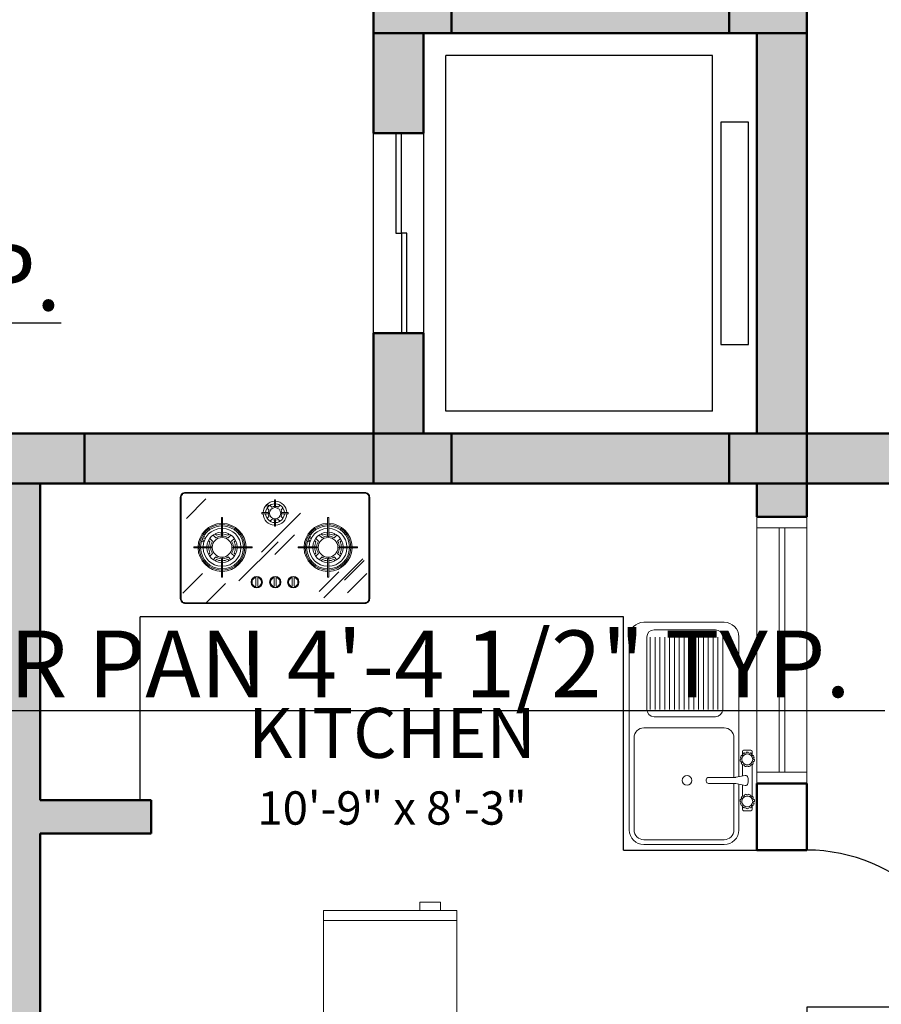
# Model space of a CAD drawing. Units: inches. Extents: x 375 to 1122, y 27 to 1069.
# Tile 79 of 155: x 790 to 945, y 400 to 577. Entities that reach past the tile are written whole.
import ezdxf

# ---------------------------------------------------------------- set-up
doc = ezdxf.new("R2010")
doc.units = ezdxf.units.IN
for name, color, linetype, lineweight in [('A-ANNO-DIMS', 2, 'Continuous', 18), ('A-AREA-IDEN', 7, 'Continuous', 18), ('A-COLS-PATT', 10, 'Continuous', 13), ('A-EQPM', 55, 'Continuous', 18), ('A-FLOR-EVTR', 40, 'Continuous', 25), ('A-FLOR-FIXT', 55, 'Continuous', 18), ('A-FLOR-MILL', 55, 'Continuous', 25), ('A-WALL-PATT', 252, 'Continuous', 13), ('Columns', 10, 'Continuous', 50), ('Doors', 150, 'Continuous', 25), ('Walls', 250, 'Continuous', 50), ('Windows', 122, 'Continuous', 18)]:
    doc.layers.add(name, color=color, linetype=linetype, lineweight=lineweight)
doc.styles.get("Standard").update_dxf_attribs({"font": 'arial.ttf'})
doc.dimstyles.new('ISO-25', dxfattribs={"dimtxt": 12, "dimasz": 2.5, "dimexe": 1.5, "dimexo": 1.5, "dimtad": 1, "dimdec": 1, "dimlunit": 3, "dimtxsty": 'Standard', "dimblk": 'ARCHTICK', "dimcen": 2.5, "dimadec": 0, "dimazin": 0, "dimtfac": 1, "dimtdec": 1, "dimtmove": 0, "dimatfit": 3, "dimfxl": 1.5, "dimfxlon": 1, "dimarcsym": 0})

# ---------------------------------------------------------------- blocks, each defined once
blk = doc.blocks.new('*U13')
for p, q in [((-30, 0), (-30, -4)), ((0, 0), (0, -4))]:
    blk.add_line(p, q)
blk.add_lwpolyline([(0, 0), (0, 30), (-1.75, 30), (-1.75, 0)], close=True)
blk.add_arc((0, 0), 30, 90, 180)
blk = doc.blocks.new('A$C659B0DF6')
for p, q in [((24, 606.07), (0, 606.07)), ((0, 585.72), (0, 606.07)), ((17.35, 607.55), (17.35, 606.07)), ((21.05, 607.55), (17.35, 607.55)), ((21.05, 606.07), (21.05, 607.55)), ((24, 585.72), (24, 606.07)), ((24, 604.22), (0, 604.22)), ((24, 585.72), (0, 585.72)), ((3.37, 583.91), (3.37, 585.72)), ((20.63, 583.91), (20.63, 585.72)), ((3.37, 583.91), (20.63, 583.91))]:
    blk.add_line(p, q)
blk = doc.blocks.new('TARJA2')
for p, q in [((-0.1232, -0.0169), (-0.1232, -0.0469)), ((-0.1182, -0.0119), (-0.1039, -0.0119)), ((-0.1122, -0.0279), (-0.1134, -0.0278)), ((-0.1122, -0.0358), (-0.1134, -0.0359)), ((-0.11, -0.0204), (-0.1111, -0.0199)), ((-0.1058, -0.0138), (-0.1067, -0.013)), ((-0.0999, -0.0087), (-0.1005, -0.0077)), ((-0.0928, -0.0055), (-0.0931, -0.0043)), ((-0.085, -0.0044), (-0.085, -0.0031)), ((-0.0773, -0.0055), (-0.0769, -0.0043)), ((-0.0701, -0.0087), (-0.0695, -0.0077)), ((-0.0642, -0.0138), (-0.0633, -0.013)), ((-0.0629, -0.0119), (0.0668, -0.0119)), ((-0.06, -0.0204), (-0.0589, -0.0199)), ((-0.0578, -0.0279), (-0.0566, -0.0278)), ((-0.0578, -0.0358), (-0.0566, -0.0359)), ((0.0617, -0.0279), (0.0605, -0.0278)), ((0.0617, -0.0358), (0.0605, -0.0359)), ((0.0639, -0.0204), (0.0628, -0.0199)), ((0.0682, -0.0138), (0.0672, -0.013)), ((0.0741, -0.0087), (0.0734, -0.0077)), ((0.0812, -0.0055), (0.0809, -0.0043)), ((0.0889, -0.0044), (0.0889, -0.0031)), ((0.0967, -0.0055), (0.097, -0.0043)), ((0.1038, -0.0087), (0.1045, -0.0077)), ((0.1221, -0.0119), (0.1078, -0.0119)), ((0.1097, -0.0138), (0.1107, -0.013)), ((0.114, -0.0204), (0.1151, -0.0199)), ((0.1162, -0.0279), (0.1174, -0.0278)), ((0.1162, -0.0358), (0.1174, -0.0359)), ((0.1271, -0.0169), (0.1271, -0.0469)), ((-0.1182, -0.0519), (-0.1039, -0.0519)), ((-0.11, -0.0433), (-0.1111, -0.0438)), ((-0.1058, -0.0499), (-0.1067, -0.0507)), ((-0.0999, -0.055), (-0.1005, -0.056)), ((-0.0928, -0.0582), (-0.0931, -0.0594)), ((-0.085, -0.0594), (-0.085, -0.0606)), ((-0.0773, -0.0582), (-0.0769, -0.0594)), ((-0.0701, -0.055), (-0.0695, -0.056)), ((-0.0642, -0.0499), (-0.0633, -0.0507)), ((-0.0629, -0.0519), (-0.0165, -0.0519)), ((-0.06, -0.0433), (-0.0589, -0.0438)), ((-0.0109, -0.0792), (-0.0187, -0.0409)), ((0.0149, -0.0792), (0.0226, -0.0409)), ((0.0204, -0.0519), (0.0668, -0.0519)), ((0.0639, -0.0433), (0.0628, -0.0438)), ((0.0682, -0.0499), (0.0672, -0.0507)), ((0.0741, -0.055), (0.0734, -0.056)), ((0.0812, -0.0582), (0.0809, -0.0594)), ((0.0889, -0.0594), (0.0889, -0.0606)), ((0.0967, -0.0582), (0.097, -0.0594)), ((0.1038, -0.055), (0.1045, -0.056)), ((0.1221, -0.0519), (0.1078, -0.0519)), ((0.1097, -0.0499), (0.1107, -0.0507)), ((0.114, -0.0433), (0.1151, -0.0438)), ((-0.0105, -0.0832), (-0.0105, -0.1919)), ((0.0145, -0.0832), (0.0145, -0.1919)), ((0.5952, -0.1334), (0.2956, -0.1334)), ((0.5952, -0.1534), (0.2956, -0.1534)), ((-0.0005, -0.2019), (0.0045, -0.2019)), ((0.2656, -0.1634), (0.2656, -0.4178)), ((0.5952, -0.1734), (0.2956, -0.1734)), ((0.5952, -0.1934), (0.2956, -0.1934)), ((0.6252, -0.4178), (0.6252, -0.1634)), ((0.5952, -0.2134), (0.2956, -0.2134)), ((0.5952, -0.2334), (0.2956, -0.2334)), ((0.5952, -0.2534), (0.2956, -0.2534)), ((0.5952, -0.2734), (0.2956, -0.2734)), ((0.5952, -0.2934), (0.2956, -0.2934)), ((0.5952, -0.3134), (0.2956, -0.3134)), ((0.5952, -0.3334), (0.2956, -0.3334)), ((0.5952, -0.3534), (0.2956, -0.3534)), ((0.5952, -0.3734), (0.2956, -0.3734)), ((0.5952, -0.3934), (0.2956, -0.3934)), ((0.5952, -0.4134), (0.2956, -0.4134)), ((0.5952, -0.4334), (0.2956, -0.4334)), ((0.2956, -0.4478), (0.5952, -0.4478))]:
    blk.add_line(p, q)
for points in [[(0.0173, -0.0671), (0.5964, -0.0671, -0.414214), (0.6564, -0.1271), (0.6564, -0.4602, -0.414214), (0.5964, -0.5202), (-0.2033, -0.5202, -0.414214), (-0.2633, -0.4602), (-0.2633, -0.1271, -0.414214)], [(-0.2633, -0.1271, -0.414214), (-0.2033, -0.0671), (-0.0134, -0.0671, -0.414214)], [(0.0145, -0.0871), (0.1793, -0.0871, -0.414214), (0.2193, -0.1271), (0.2193, -0.4602, -0.414214), (0.1793, -0.5002), (-0.2033, -0.5002, -0.414214), (-0.2433, -0.4602), (-0.2433, -0.1271, -0.414214)], [(-0.2433, -0.1271, -0.414214), (-0.2033, -0.0871), (-0.0105, -0.0871, -0.414214)]]:
    blk.add_lwpolyline(points, format="xyb")
for centre, radius in [((-0.085, -0.0319), 0.0225), ((0.0889, -0.0319), 0.0225), ((0.002, -0.2812), 0.02)]:
    blk.add_circle(centre, radius)
for centre, radius, start, end in [((-0.1182, -0.0169), 0.005, 90, 180), ((-0.085, -0.0319), 0.03, 174.3101, 185.6899), ((-0.1136, -0.029), 0.00125, 81.8182, 174.3101), ((-0.1136, -0.0347), 0.00125, 185.6899, 278.1818), ((-0.085, -0.0319), 0.0275, 155.4545, 171.8182), ((-0.085, -0.0319), 0.0275, 188.1818, 204.5455), ((-0.1106, -0.0188), 0.00125, 152.9626, 245.4545), ((-0.085, -0.0319), 0.03, 141.5828, 152.9626), ((-0.1075, -0.014), 0.00125, 49.0909, 141.5828), ((-0.085, -0.0319), 0.0275, 122.7273, 139.0909), ((-0.0995, -0.007), 0.00125, 120.2354, 212.7273), ((-0.085, -0.0319), 0.03, 108.8555, 120.2354), ((-0.0943, -0.0046), 0.00125, 16.3636, 108.8555), ((-0.085, -0.0319), 0.0275, 90, 106.3636), ((-0.0838, -0.0031), 0.00125, 87.5081, 180), ((-0.085, -0.0319), 0.03, 76.1283, 87.5081), ((-0.0781, -0.0039), 0.00125, 343.6364, 76.1283), ((-0.085, -0.0319), 0.0275, 57.2727, 73.6364), ((-0.0684, -0.0084), 0.00125, 54.7808, 147.2727), ((-0.085, -0.0319), 0.03, 43.401, 54.7808), ((-0.085, -0.0319), 0.0275, 24.5455, 40.9091), ((-0.0641, -0.0121), 0.00125, 310.9091, 43.401), ((-0.0584, -0.0211), 0.00125, 22.0535, 114.5455), ((-0.085, -0.0319), 0.0275, 351.8182, 8.1818), ((-0.085, -0.0319), 0.03, 10.6737, 22.0535), ((-0.085, -0.0319), 0.03, 337.9465, 349.3263), ((-0.0568, -0.0265), 0.00125, 278.1818, 10.6737), ((-0.0568, -0.0372), 0.00125, 349.3263, 81.8182), ((-0.0089, -0.039), 0.01, 101.1605, 191.4527), ((0.002, -0.094), 0.0661, 78.8395, 101.1605), ((0.0128, -0.039), 0.01, 348.5473, 78.8395), ((0.0607, -0.0265), 0.00125, 169.3263, 261.8182), ((0.0607, -0.0372), 0.00125, 98.1818, 190.6737), ((0.0889, -0.0319), 0.03, 157.9465, 169.3263), ((0.0889, -0.0319), 0.03, 190.6737, 202.0535), ((0.0623, -0.0211), 0.00125, 65.4545, 157.9465), ((0.0889, -0.0319), 0.0275, 171.8182, 188.1818), ((0.0889, -0.0319), 0.0275, 139.0909, 155.4545), ((0.0681, -0.0121), 0.00125, 136.599, 229.0909), ((0.0889, -0.0319), 0.03, 125.2192, 136.599), ((0.0724, -0.0084), 0.00125, 32.7273, 125.2192), ((0.0889, -0.0319), 0.0275, 106.3636, 122.7273), ((0.0821, -0.0039), 0.00125, 103.8717, 196.3636), ((0.0889, -0.0319), 0.03, 92.4919, 103.8717), ((0.0877, -0.0031), 0.00125, 0, 92.4919), ((0.0889, -0.0319), 0.0275, 73.6364, 90), ((0.0982, -0.0046), 0.00125, 71.1445, 163.6364), ((0.0889, -0.0319), 0.03, 59.7646, 71.1445), ((0.0889, -0.0319), 0.0275, 40.9091, 57.2727), ((0.1034, -0.007), 0.00125, 327.2727, 59.7646), ((0.1115, -0.014), 0.00125, 38.4172, 130.9091), ((0.0889, -0.0319), 0.03, 27.0374, 38.4172), ((0.0889, -0.0319), 0.0275, 8.1818, 24.5455), ((0.0889, -0.0319), 0.0275, 335.4545, 351.8182), ((0.1146, -0.0188), 0.00125, 294.5455, 27.0374), ((0.1176, -0.029), 0.00125, 5.6899, 98.1818), ((0.1176, -0.0347), 0.00125, 261.8182, 354.3101), ((0.0889, -0.0319), 0.03, 354.3101, 5.6899), ((0.1221, -0.0169), 0.005, 0, 90), ((-0.1182, -0.0469), 0.005, 180, 270), ((-0.1106, -0.0449), 0.00125, 114.5455, 207.0374), ((-0.085, -0.0319), 0.03, 207.0374, 218.4172), ((-0.1075, -0.0497), 0.00125, 218.4172, 310.9091), ((-0.085, -0.0319), 0.0275, 220.9091, 237.2727), ((-0.0995, -0.0567), 0.00125, 147.2727, 239.7646), ((-0.085, -0.0319), 0.03, 239.7646, 251.1445), ((-0.0943, -0.0591), 0.00125, 251.1445, 343.6364), ((-0.085, -0.0319), 0.0275, 253.6364, 270), ((-0.0838, -0.0606), 0.00125, 180, 272.4919), ((-0.085, -0.0319), 0.03, 272.4919, 283.8717), ((-0.0781, -0.0598), 0.00125, 283.8717, 16.3636), ((-0.085, -0.0319), 0.0275, 286.3636, 302.7273), ((-0.0684, -0.0553), 0.00125, 212.7273, 305.2192), ((-0.085, -0.0319), 0.03, 305.2192, 316.599), ((-0.085, -0.0319), 0.0275, 319.0909, 335.4545), ((-0.0641, -0.0516), 0.00125, 316.599, 49.0909), ((-0.0584, -0.0426), 0.00125, 245.4545, 337.9465), ((-0.0305, -0.0832), 0.02, 0, 11.4527), ((-0.0205, -0.0822), 0.01, 0, 11.4527), ((0.0345, -0.0832), 0.02, 168.5473, 180), ((0.0623, -0.0426), 0.00125, 202.0535, 294.5455), ((0.0889, -0.0319), 0.0275, 204.5455, 220.9091), ((0.0681, -0.0516), 0.00125, 130.9091, 223.401), ((0.0889, -0.0319), 0.03, 223.401, 234.7808), ((0.0724, -0.0553), 0.00125, 234.7808, 327.2727), ((0.0889, -0.0319), 0.0275, 237.2727, 253.6364), ((0.0821, -0.0598), 0.00125, 163.6364, 256.1283), ((0.0889, -0.0319), 0.03, 256.1283, 267.5081), ((0.0877, -0.0606), 0.00125, 267.5081, 360), ((0.0889, -0.0319), 0.0275, 270, 286.3636), ((0.0982, -0.0591), 0.00125, 196.3636, 288.8555), ((0.0889, -0.0319), 0.03, 288.8555, 300.2354), ((0.0889, -0.0319), 0.0275, 302.7273, 319.0909), ((0.1034, -0.0567), 0.00125, 300.2354, 32.7273), ((0.1115, -0.0497), 0.00125, 229.0909, 321.5828), ((0.0889, -0.0319), 0.03, 321.5828, 332.9626), ((0.1146, -0.0449), 0.00125, 332.9626, 65.4545), ((0.1221, -0.0469), 0.005, 270, 360), ((0.2956, -0.1634), 0.03, 90, 180), ((0.5952, -0.1634), 0.03, 0, 90), ((-0.0005, -0.1919), 0.01, 180, 270), ((0.0045, -0.1919), 0.01, 270, 360), ((0.2956, -0.4178), 0.03, 180, 270), ((0.5952, -0.4178), 0.03, 270, 360)]:
    blk.add_arc(centre, radius, start, end)
blk = doc.blocks.new('A$C42203764')
at = {"xscale": 1000, "yscale": 1000, "zscale": 1000}
blk.add_blockref('TARJA2', (263.3, 520.2), dxfattribs=at)
blk = doc.blocks.new('A$C038F079D')
for p, q in [((23.9, 336.8), (101.3, 414.2)), ((377.5, 410.6), (372.5, 410.6)), ((320.9, 202.7), (475.7, 357.5)), ((427.1, 359.8), (427.1, 354.8)), ((587.4, 339.9), (582.4, 339.9)), ((377.5, 305.6), (372.5, 305.6)), ((232.1, 89.3), (386.9, 244.1)), ((374.2, 193.8), (451.6, 271.2)), ((53.2, 224.7), (53.2, 219.7)), ((284, 224.7), (284, 219.7)), ((466, 224.7), (466, 219.7)), ((701.8, 224.7), (701.8, 219.7)), ((130.3, 173.3), (141.1, 184.1)), ((137.3, 169), (142.6, 174.2)), ((567.6, 22.2), (722.4, 177)), ((650.5, 92.2), (727.9, 169.6)), ((10.1, 41), (87.5, 118.4)), ((549.9, 47.9), (627.2, 125.3)), ((661.4, 42), (738.7, 119.3)), ((100.9, 1.5), (178.3, 78.9)), ((587.4, 103.7), (582.4, 103.7))]:
    blk.add_line(p, q)
at = {"ltscale": 0.18}
for p, q in [((372.5, 384.7), (372.5, 410.6)), ((377.5, 384.7), (377.5, 410.6)), ((322.3, 354.8), (322.3, 359.8)), ((347.6, 359.8), (322.3, 359.8)), ((347.6, 354.8), (322.3, 354.8)), ((350.8, 370.2), (343.5, 377.5)), ((362.2, 381.5), (354.8, 388.8)), ((387.8, 381.5), (395.2, 388.8)), ((399.2, 370.2), (406.5, 377.5)), ((402.4, 359.8), (427.1, 359.8)), ((402.4, 354.8), (427.1, 354.8)), ((162.6, 339.9), (167.6, 339.9)), ((162.6, 267.1), (162.6, 339.9)), ((167.6, 267.1), (167.6, 339.9)), ((343.5, 337.2), (350.8, 344.5)), ((354.8, 325.8), (362.2, 333.1)), ((372.5, 329.9), (372.5, 305.6)), ((377.5, 329.9), (377.5, 305.6)), ((395.2, 325.8), (387.8, 333.1)), ((406.5, 337.2), (399.2, 344.5)), ((582.4, 267.1), (582.4, 339.9)), ((587.4, 267.1), (587.4, 339.9)), ((137.3, 275.4), (142.6, 270.2)), ((187.6, 270.2), (192.8, 275.4)), ((562.4, 270.2), (557.2, 275.4)), ((612.7, 275.4), (607.4, 270.2)), ((111.9, 250), (117.1, 244.7)), ((116.2, 257), (127, 246.2)), ((130.3, 271.1), (141.1, 260.3)), ((189, 260.3), (199.8, 271.1)), ((203.2, 246.2), (214, 257)), ((213.1, 244.7), (218.3, 250)), ((536.9, 244.7), (531.7, 250)), ((546.8, 246.2), (536, 257)), ((561, 260.3), (550.2, 271.1)), ((619.7, 271.1), (608.9, 260.3)), ((633.8, 257), (623, 246.2)), ((638.1, 250), (632.9, 244.7)), ((125.1, 224.7), (53.2, 224.7)), ((125.1, 219.7), (53.2, 219.7)), ((111.9, 194.5), (117.1, 199.7)), ((116.2, 187.5), (127, 198.3)), ((203.2, 198.3), (214, 187.5)), ((210, 224.7), (284, 224.7)), ((210, 219.7), (284, 219.7)), ((213.1, 199.7), (218.3, 194.5)), ((540, 224.7), (466, 224.7)), ((540, 219.7), (466, 219.7)), ((536.9, 199.7), (531.7, 194.5)), ((546.8, 198.3), (536, 187.5)), ((633.8, 187.5), (623, 198.3)), ((629.9, 224.7), (701.8, 224.7)), ((629.9, 219.7), (701.8, 219.7)), ((638.1, 194.5), (632.9, 199.7)), ((162.6, 177.3), (162.6, 103.7)), ((167.6, 177.3), (167.6, 103.7)), ((187.6, 174.2), (192.8, 169)), ((189, 184.1), (199.8, 173.3)), ((561, 184.1), (550.2, 173.3)), ((562.4, 174.2), (557.2, 169)), ((582.4, 177.3), (582.4, 103.7)), ((587.4, 177.3), (587.4, 103.7)), ((612.7, 169), (607.4, 174.2)), ((619.7, 173.3), (608.9, 184.1)), ((162.6, 103.7), (167.6, 103.7)), ((298.6, 99.8), (298.6, 69)), ((306.6, 99.8), (306.6, 69)), ((372, 99.8), (372, 69)), ((380, 99.8), (380, 69)), ((443.4, 99.8), (443.4, 69)), ((451.4, 99.8), (451.4, 69))]:
    blk.add_line(p, q, dxfattribs=at)
for points in [[(20, 0), (730, 0, 0.414214), (750, 20), (750, 420, 0.414214), (730, 440), (20, 440, 0.414214), (0, 420), (0, 20, 0.414214)], [(20, 3), (730, 3, 0.414214), (747, 20), (747, 420, 0.414214), (730, 437), (20, 437, 0.414214), (3, 420), (3, 20, 0.414214)]]:
    blk.add_lwpolyline(points, format="xyb", close=True)
for centre in [(345.9, 386.3), (89.1, 248.3), (94.7, 261.5), (509, 247.6), (514.6, 260.8)]:
    blk.add_circle(centre, 3.73)
for centre, radius in [((375, 357.3), 22.4), ((165.1, 222.2), 39), ((584.9, 222.2), 39), ((302.6, 84.4), 22.5), ((302.6, 84.4), 21.5), ((376, 84.4), 22.5), ((376, 84.4), 21.5), ((447.4, 84.4), 22.5), ((447.4, 84.4), 21.5)]:
    blk.add_circle(centre, radius, dxfattribs=at)
for centre, radius, start, end in [((375, 357.3), 47.4, 93.0255, 176.9745), ((375, 357.3), 37.4, 93.8363, 176.1637), ((375, 357.3), 47.4, 3.0255, 86.9745), ((375, 357.3), 37.4, 3.8363, 86.1637), ((375, 357.3), 47.4, 183.0255, 266.9745), ((375, 357.3), 37.4, 183.8363, 266.1637), ((346.8, 357.3), 2.62, 287.6318, 72.3682), ((375, 357.3), 27.4, 151.9979, 174.8384), ((375, 357.3), 27.4, 185.1616, 208.0021), ((375, 357.3), 27.4, 95.203, 118.0021), ((375, 385), 2.52, 187.9505, 352.0495), ((375, 357.3), 27.4, 61.9979, 84.797), ((375, 357.3), 47.4, 273.0255, 356.9745), ((375, 357.3), 37.4, 273.8363, 356.1637), ((375, 357.3), 27.4, 5.206, 28.0021), ((375, 357.3), 27.4, 331.9979, 354.794), ((402.7, 357.3), 2.52, 97.2236, 262.7764), ((165.1, 222.2), 95, 91.5918, 178.4082), ((165.1, 222.2), 90, 91.5918, 178.4082), ((165.1, 222.2), 90, 1.5918, 88.4082), ((165.1, 222.2), 95, 1.5918, 88.4082), ((375, 357.3), 27.4, 241.9979, 264.7569), ((375, 330), 2.5, 358.3317, 181.6683), ((375, 357.3), 27.4, 275.2431, 298.0021), ((584.9, 222.2), 95, 91.5918, 178.4082), ((584.9, 222.2), 90, 91.5918, 178.4082), ((584.9, 222.2), 90, 1.5918, 88.4082), ((584.9, 222.2), 95, 1.5918, 88.4082), ((165.1, 222.2), 85, 91.6854, 178.3146), ((165.1, 222.2), 75, 91.9102, 178.0898), ((165.1, 222.2), 60, 92.388, 177.612), ((165.1, 222.2), 53, 92.7036, 115.1461), ((165.1, 222.2), 85, 1.6854, 88.3146), ((165.1, 222.2), 75, 1.9102, 88.0898), ((165.1, 222.2), 60, 2.388, 87.612), ((165.1, 222.2), 53, 64.8539, 87.2964), ((584.9, 222.2), 85, 91.6854, 178.3146), ((584.9, 222.2), 75, 91.9102, 178.0898), ((584.9, 222.2), 60, 92.388, 177.612), ((584.9, 222.2), 53, 92.7036, 115.1461), ((584.9, 222.2), 85, 1.6854, 88.3146), ((584.9, 222.2), 75, 1.9102, 88.0898), ((584.9, 222.2), 60, 2.388, 87.612), ((584.9, 222.2), 53, 64.8539, 87.2964), ((165.1, 222.2), 53, 154.8539, 177.2964), ((165.1, 222.2), 45, 147.8396, 176.8153), ((165.1, 222.2), 45, 93.1847, 122.1604), ((165.1, 267.4), 2.52, 186.7354, 353.2646), ((165.1, 222.2), 45, 57.8396, 86.8153), ((165.1, 222.2), 45, 3.1847, 32.1604), ((165.1, 222.2), 53, 2.7036, 25.1461), ((584.9, 222.2), 53, 154.8539, 177.2964), ((584.9, 222.2), 45, 147.8396, 176.8153), ((584.9, 222.2), 45, 93.1847, 122.1604), ((584.9, 267.3), 2.51, 183.9579, 356.0421), ((584.9, 222.2), 45, 57.8396, 86.8153), ((584.9, 222.2), 45, 3.1847, 32.1604), ((584.9, 222.2), 53, 2.7036, 25.1461), ((165.1, 222.2), 95, 181.5918, 268.4082), ((165.1, 222.2), 90, 181.5918, 268.4082), ((165.1, 222.2), 85, 181.6854, 268.3146), ((165.1, 222.2), 75, 181.9102, 268.0898), ((165.1, 222.2), 60, 182.388, 267.612), ((165.1, 222.2), 53, 182.7036, 205.1461), ((119.3, 222.2), 2.64, 288.751, 71.249), ((165.1, 222.2), 45, 183.1847, 212.1604), ((165.1, 222.2), 75, 271.9102, 358.0898), ((165.1, 222.2), 60, 272.388, 357.612), ((165.1, 222.2), 85, 271.6854, 358.3146), ((165.1, 222.2), 90, 271.5918, 358.4082), ((165.1, 222.2), 95, 271.5918, 358.4082), ((165.1, 222.2), 45, 327.8396, 356.8153), ((210.9, 222.2), 2.67, 110.5507, 249.4493), ((165.1, 222.2), 53, 334.8539, 357.2964), ((584.9, 222.2), 95, 181.5918, 268.4082), ((584.9, 222.2), 90, 181.5918, 268.4082), ((584.9, 222.2), 85, 181.6854, 268.3146), ((584.9, 222.2), 75, 181.9102, 268.0898), ((584.9, 222.2), 60, 182.388, 267.612), ((584.9, 222.2), 53, 182.7036, 205.1461), ((539.2, 222.2), 2.63, 288.412, 71.588), ((584.9, 222.2), 45, 183.1847, 212.1604), ((584.9, 222.2), 90, 271.5918, 358.4082), ((584.9, 222.2), 85, 271.6854, 358.3146), ((584.9, 222.2), 75, 271.9102, 358.0898), ((584.9, 222.2), 60, 272.388, 357.612), ((584.9, 222.2), 95, 271.5918, 358.4082), ((584.9, 222.2), 45, 327.8396, 356.8153), ((630.5, 222.2), 2.58, 104.2945, 255.7055), ((584.9, 222.2), 53, 334.8539, 357.2964), ((165.1, 222.2), 45, 237.8396, 266.8153), ((165.1, 222.2), 53, 244.8539, 267.2964), ((165.1, 222.2), 45, 273.1847, 302.1604), ((165.1, 222.2), 53, 272.7036, 295.1461), ((584.9, 222.2), 45, 237.8396, 266.8153), ((584.9, 222.2), 53, 244.8539, 267.2964), ((584.9, 176.5), 2.63, 17.9418, 162.0582), ((584.9, 222.2), 45, 273.1847, 302.1604), ((584.9, 222.2), 53, 272.7036, 295.1461), ((302.6, 84.4), 18.5, 111.3237, 248.6763), ((296.6, 99.8), 2, 0, 111.3237), ((308.6, 99.8), 2, 68.6763, 180), ((302.6, 84.4), 18.5, 291.3237, 68.6763), ((376, 84.4), 18.5, 111.3237, 248.6763), ((370, 99.8), 2, 0, 111.3237), ((382, 99.8), 2, 68.6763, 180), ((376, 84.4), 18.5, 291.3237, 68.6763), ((447.4, 84.4), 18.5, 111.3237, 248.6763), ((441.4, 99.8), 2, 0, 111.3237), ((453.4, 99.8), 2, 68.6763, 180), ((447.4, 84.4), 18.5, 291.3237, 68.6763), ((296.6, 69), 2, 248.6763, 0), ((308.6, 69), 2, 180, 291.3237), ((370, 69), 2, 248.6763, 0), ((382, 69), 2, 180, 291.3237), ((441.4, 69), 2, 248.6763, 0), ((453.4, 69), 2, 180, 291.3237)]:
    blk.add_arc(centre, radius, start, end, dxfattribs=at)
blk.add_arc((165.1, 176.3), 2.69, 21.7885, 158.2115)
blk = doc.blocks.new('WINDOW-48IN')
for p, q in [((2, 5), (46, 5)), ((2, 4), (46, 4))]:
    blk.add_line(p, q)
blk.add_lwpolyline([(48, 0), (0, 0), (0, 9), (48, 9)], close=True)
for points in [[(2, 0), (2, 9)], [(46, 9), (46, 0)]]:
    blk.add_lwpolyline(points)
blk = doc.blocks.new('COLUMN-14X9IN')
blk.add_lwpolyline([(0, 0), (14, 0), (14, 9), (0, 9)], close=True)
blk = doc.blocks.new('KITCHEN-COUNTER-L')
for p, q in [((0, 9), (0, 42)), ((87, 42), (0, 42)), ((87, 0), (87, 42)), ((87, 0), (111, 0))]:
    blk.add_line(p, q)
blk = doc.blocks.new('_ArchTick')
at = {"color": 0, "linetype": 'ByBlock', "const_width": 0.15}
blk.add_lwpolyline([(-0.5, -0.5), (0.5, 0.5)], dxfattribs=at)
blk = doc.blocks.new('*D52')
at = {"layer": 'A-ANNO-DIMS', "color": 0, "lineweight": -2, "transparency": 16777216}
for p, q in [((708.04, 521.53), (708.04, 523.93)), ((722.01, 521.53), (722.01, 523.93)), ((708.04, 522.43), (722.01, 522.43)), ((722.01, 522.43), (797.77, 522.43))]:
    blk.add_line(p, q, dxfattribs=at)
at = {"layer": 'Defpoints', "color": 0, "transparency": 16777216}
for p in [(722.01, 522.43), (708.04, 520.03), (722.01, 520.03)]:
    blk.add_point(p, dxfattribs=at)
at = {"layer": 'A-ANNO-DIMS', "color": 0, "lineweight": -2, "transparency": 16777216, "xscale": 2.5, "yscale": 2.5, "zscale": 2.5, "rotation": 180}
blk.add_blockref('_ArchTick', (708.04, 522.43), dxfattribs=at)
at = {"layer": 'A-ANNO-DIMS', "color": 0, "lineweight": -2, "transparency": 16777216, "xscale": 2.5, "yscale": 2.5, "zscale": 2.5}
blk.add_blockref('_ArchTick', (722.01, 522.43), dxfattribs=at)
at = {"layer": 'A-ANNO-DIMS', "color": 0, "transparency": 16777216, "insert": (761.14, 529.08), "char_height": 12, "attachment_point": 5}
blk.add_mtext('1\'-2" TYP.', dxfattribs=at)
blk = doc.blocks.new('*D53')
at = {"layer": 'A-ANNO-DIMS', "color": 0, "lineweight": -2, "transparency": 16777216}
for p, q in [((669.51, 454.15), (669.51, 451.15)), ((722.01, 454.15), (722.01, 451.15)), ((669.51, 452.65), (722.01, 452.65)), ((722.01, 452.65), (946.03, 452.65))]:
    blk.add_line(p, q, dxfattribs=at)
at = {"layer": 'Defpoints', "color": 0, "transparency": 16777216}
for p in [(669.51, 460.53), (722.01, 460.53), (722.01, 452.65)]:
    blk.add_point(p, dxfattribs=at)
at = {"layer": 'A-ANNO-DIMS', "color": 0, "lineweight": -2, "transparency": 16777216, "xscale": 2.5, "yscale": 2.5, "zscale": 2.5, "rotation": 180}
blk.add_blockref('_ArchTick', (669.51, 452.65), dxfattribs=at)
at = {"layer": 'A-ANNO-DIMS', "color": 0, "lineweight": -2, "transparency": 16777216, "xscale": 2.5, "yscale": 2.5, "zscale": 2.5}
blk.add_blockref('_ArchTick', (722.01, 452.65), dxfattribs=at)
at = {"layer": 'A-ANNO-DIMS', "color": 0, "transparency": 16777216, "insert": (835.27, 459.49), "char_height": 12, "attachment_point": 5}
blk.add_mtext('SHOWER PAN 4\'-4 1/2" TYP.', dxfattribs=at)
blk = doc.blocks.new('*D84')
at = {"layer": 'A-ANNO-DIMS', "color": 0, "lineweight": -2, "transparency": 16777216}
for p, q in [((845.01, 117.53), (845.01, 114.53)), ((950.01, 117.53), (950.01, 114.53)), ((845.01, 116.03), (950.01, 116.03))]:
    blk.add_line(p, q, dxfattribs=at)
at = {"layer": 'Defpoints', "color": 0, "transparency": 16777216}
for p in [(845.01, 814.53), (950.01, 814.53), (950.01, 116.03)]:
    blk.add_point(p, dxfattribs=at)
at = {"layer": 'A-ANNO-DIMS', "color": 0, "lineweight": -2, "transparency": 16777216, "xscale": 2.5, "yscale": 2.5, "zscale": 2.5, "rotation": 180}
blk.add_blockref('_ArchTick', (845.01, 116.03), dxfattribs=at)
at = {"layer": 'A-ANNO-DIMS', "color": 0, "lineweight": -2, "transparency": 16777216, "xscale": 2.5, "yscale": 2.5, "zscale": 2.5}
blk.add_blockref('_ArchTick', (950.01, 116.03), dxfattribs=at)
at = {"layer": 'A-ANNO-DIMS', "color": 0, "transparency": 16777216, "insert": (897.51, 122.78), "char_height": 12, "attachment_point": 5}
blk.add_mtext('8\'-9"', dxfattribs=at)
blk = doc.blocks.new('*D87')
at = {"layer": 'A-ANNO-DIMS', "color": 0, "lineweight": -2, "transparency": 16777216}
for p, q in [((794.01, 117.53), (794.01, 114.53)), ((884.01, 117.53), (884.01, 114.53)), ((794.01, 116.03), (884.01, 116.03))]:
    blk.add_line(p, q, dxfattribs=at)
at = {"layer": 'Defpoints', "color": 0, "transparency": 16777216}
for p in [(794.01, 583.53), (884.01, 583.53), (884.01, 116.03)]:
    blk.add_point(p, dxfattribs=at)
at = {"layer": 'A-ANNO-DIMS', "color": 0, "lineweight": -2, "transparency": 16777216, "xscale": 2.5, "yscale": 2.5, "zscale": 2.5, "rotation": 180}
blk.add_blockref('_ArchTick', (794.01, 116.03), dxfattribs=at)
at = {"layer": 'A-ANNO-DIMS', "color": 0, "lineweight": -2, "transparency": 16777216, "xscale": 2.5, "yscale": 2.5, "zscale": 2.5}
blk.add_blockref('_ArchTick', (884.01, 116.03), dxfattribs=at)
at = {"layer": 'A-ANNO-DIMS', "color": 0, "transparency": 16777216, "insert": (839.01, 122.78), "char_height": 12, "attachment_point": 5}
blk.add_mtext('7\'-6"', dxfattribs=at)
blk = doc.blocks.new('*D88')
at = {"layer": 'A-ANNO-DIMS', "color": 0, "lineweight": -2, "transparency": 16777216}
for p, q in [((731.01, 1052.53), (731.01, 1055.53)), ((854.01, 1052.53), (854.01, 1055.53)), ((731.01, 1054.03), (854.01, 1054.03))]:
    blk.add_line(p, q, dxfattribs=at)
at = {"layer": 'Defpoints', "color": 0, "transparency": 16777216}
for p in [(854.01, 1054.03), (731.01, 502.53), (854.01, 502.53)]:
    blk.add_point(p, dxfattribs=at)
at = {"layer": 'A-ANNO-DIMS', "color": 0, "lineweight": -2, "transparency": 16777216, "xscale": 2.5, "yscale": 2.5, "zscale": 2.5, "rotation": 180}
blk.add_blockref('_ArchTick', (731.01, 1054.03), dxfattribs=at)
at = {"layer": 'A-ANNO-DIMS', "color": 0, "lineweight": -2, "transparency": 16777216, "xscale": 2.5, "yscale": 2.5, "zscale": 2.5}
blk.add_blockref('_ArchTick', (854.01, 1054.03), dxfattribs=at)
at = {"layer": 'A-ANNO-DIMS', "color": 0, "transparency": 16777216, "insert": (792.51, 1060.78), "char_height": 12, "attachment_point": 5}
blk.add_mtext('10\'-3"', dxfattribs=at)
blk = doc.blocks.new('*D89')
at = {"layer": 'A-ANNO-DIMS', "color": 0, "lineweight": -2, "transparency": 16777216}
for p, q in [((863.01, 117.53), (863.01, 114.53)), ((923.01, 117.53), (923.01, 114.53)), ((863.01, 116.03), (923.01, 116.03))]:
    blk.add_line(p, q, dxfattribs=at)
at = {"layer": 'Defpoints', "color": 0, "transparency": 16777216}
for p in [(863.01, 574.53), (923.01, 574.53), (923.01, 116.03)]:
    blk.add_point(p, dxfattribs=at)
at = {"layer": 'A-ANNO-DIMS', "color": 0, "lineweight": -2, "transparency": 16777216, "xscale": 2.5, "yscale": 2.5, "zscale": 2.5, "rotation": 180}
blk.add_blockref('_ArchTick', (863.01, 116.03), dxfattribs=at)
at = {"layer": 'A-ANNO-DIMS', "color": 0, "lineweight": -2, "transparency": 16777216, "xscale": 2.5, "yscale": 2.5, "zscale": 2.5}
blk.add_blockref('_ArchTick', (923.01, 116.03), dxfattribs=at)
at = {"layer": 'A-ANNO-DIMS', "color": 0, "transparency": 16777216, "insert": (893.01, 122.78), "char_height": 12, "attachment_point": 5}
blk.add_mtext('5\'-0"', dxfattribs=at)
blk = doc.blocks.new('*D90')
at = {"layer": 'A-ANNO-DIMS', "color": 0, "lineweight": -2, "transparency": 16777216}
for p, q in [((401.51, 574.53), (398.51, 574.53)), ((400.01, 502.53), (400.01, 574.53)), ((401.51, 502.53), (398.51, 502.53))]:
    blk.add_line(p, q, dxfattribs=at)
at = {"layer": 'Defpoints', "color": 0, "transparency": 16777216}
for p in [(400.01, 574.53), (863.01, 574.53), (863.01, 502.53)]:
    blk.add_point(p, dxfattribs=at)
at = {"layer": 'A-ANNO-DIMS', "color": 0, "lineweight": -2, "transparency": 16777216, "xscale": 2.5, "yscale": 2.5, "zscale": 2.5}
for p, rotation in [((400.01, 574.53), 90), ((400.01, 502.53), 270)]:
    blk.add_blockref('_ArchTick', p, dxfattribs=dict(at, rotation=rotation))
at = {"layer": 'A-ANNO-DIMS', "color": 0, "transparency": 16777216, "insert": (393.26, 538.53), "char_height": 12, "attachment_point": 5, "rotation": 90}
blk.add_mtext('6\'-0"', dxfattribs=at)

msp = doc.modelspace()

# ---------------------------------------------------------------- hatches: boundary and pattern name
at = {"layer": 'A-COLS-PATT'}
h = msp.add_hatch(color=256, dxfattribs=at)
h.dxf.hatch_style = 1
h.paths.add_polyline_path([(512.51, 982.53), (498.51, 982.53), (498.51, 973.53), (512.51, 973.53)])
h.paths.add_polyline_path([(666.51, 982.53), (652.51, 982.53), (652.51, 973.53), (666.51, 973.53)])
h.paths.add_polyline_path([(802.01, 982.53), (788.01, 982.53), (788.01, 973.53), (802.01, 973.53)])
h.paths.add_polyline_path([(932.01, 982.53), (918.01, 982.53), (918.01, 973.53), (932.01, 973.53)])
h.paths.add_polyline_path([(507.51, 841.53), (498.51, 841.53), (498.51, 827.53), (507.51, 827.53)])
h.paths.add_polyline_path([(666.51, 844.53), (652.51, 844.53), (652.51, 835.53), (666.51, 835.53)])
h.paths.add_polyline_path([(802.01, 814.53), (788.01, 814.53), (788.01, 805.53), (802.01, 805.53)])
h.paths.add_polyline_path([(932.01, 814.53), (918.01, 814.53), (918.01, 805.53), (932.01, 805.53)])
h.paths.add_polyline_path([(507.51, 719.53), (498.51, 719.53), (498.51, 705.53), (507.51, 705.53)])
h.paths.add_polyline_path([(731.01, 676.53), (722.01, 676.53), (722.01, 662.53), (731.01, 662.53)])
h.paths.add_polyline_path([(802.01, 676.53), (788.01, 676.53), (788.01, 667.53), (802.01, 667.53)])
h.paths.add_polyline_path([(932.01, 676.53), (918.01, 676.53), (918.01, 667.53), (932.01, 667.53)])
h.paths.add_polyline_path([(932.01, 583.53), (918.01, 583.53), (918.01, 574.53), (932.01, 574.53)])
h.paths.add_polyline_path([(868.01, 583.53), (854.01, 583.53), (854.01, 574.53), (868.01, 574.53)])
h.paths.add_polyline_path([(868.01, 502.53), (854.01, 502.53), (854.01, 493.53), (868.01, 493.53)])
h.paths.add_polyline_path([(932.01, 502.53), (918.01, 502.53), (918.01, 493.53), (932.01, 493.53)])
h.paths.add_polyline_path([(672.51, 592.03), (663.51, 592.03), (663.51, 578.03), (672.51, 578.03)])
h.paths.add_polyline_path([(512.51, 589.53), (498.51, 589.53), (498.51, 580.53), (512.51, 580.53)])
h.paths.add_polyline_path([(507.51, 464.53), (498.51, 464.53), (498.51, 450.53), (507.51, 450.53)])
h.paths.add_polyline_path([(731.01, 507.53), (722.01, 507.53), (722.01, 493.53), (731.01, 493.53)])
h.paths.add_polyline_path([(802.01, 502.53), (788.01, 502.53), (788.01, 493.53), (802.01, 493.53)])
h.paths.add_polyline_path([(507.51, 342.53), (498.51, 342.53), (498.51, 328.53), (507.51, 328.53)])
h.paths.add_polyline_path([(512.51, 196.53), (498.51, 196.53), (498.51, 187.53), (512.51, 187.53)])
h.paths.add_polyline_path([(666.51, 334.53), (652.51, 334.53), (652.51, 325.53), (666.51, 325.53)])
h.paths.add_polyline_path([(666.51, 196.53), (652.51, 196.53), (652.51, 187.53), (666.51, 187.53)])
h.paths.add_polyline_path([(805.01, 196.53), (791.01, 196.53), (791.01, 187.53), (805.01, 187.53)])
h.paths.add_polyline_path([(932.01, 196.53), (918.01, 196.53), (918.01, 187.53), (932.01, 187.53)])
h.paths.add_polyline_path([(932.01, 334.53), (918.01, 334.53), (918.01, 325.53), (932.01, 325.53)])
h.paths.add_polyline_path([(805.01, 334.53), (791.01, 334.53), (791.01, 325.53), (805.01, 325.53)])
at = {"layer": 'A-WALL-PATT'}
h = msp.add_hatch(color=256, dxfattribs=at)
h.dxf.hatch_style = 1
h.paths.add_polyline_path([(962.01, 388.53), (989.01, 388.53), (989.01, 394.53), (962.01, 394.53), (932.01, 394.53), (932.01, 397.53), (923.01, 397.53), (923.01, 394.53), (842.01, 394.53), (842.01, 334.53), (839.51, 334.53), (839.51, 328.53), (854.01, 328.53), (854.01, 334.53), (848.01, 334.53), (848.01, 388.53), (953.01, 388.53), (953.01, 356.08), (962.01, 356.08), (962.01, 358.55), (989.01, 358.55), (989.01, 364.55), (962.01, 364.55)])
h.paths.add_polyline_path([(989.01, 502.53), (932.01, 502.53), (932.01, 583.53), (932.01, 593.53), (923.01, 593.53), (923.01, 583.53), (854.01, 583.53), (854.01, 556.53), (863.01, 556.53), (863.01, 574.53), (923.01, 574.53), (923.01, 502.53), (863.01, 502.53), (863.01, 520.53), (854.01, 520.53), (854.01, 502.53), (773.01, 502.53), (773.01, 493.53), (788.01, 493.53), (788.01, 402.03), (722.01, 402.03), (722.01, 373.53), (728.01, 373.53), (728.01, 396.03), (788.01, 396.03), (788.01, 373.53), (794.01, 373.53), (794.01, 430.53), (814.01, 430.53), (814.01, 436.53), (794.01, 436.53), (794.01, 493.53), (923.01, 493.53), (923.01, 487.53), (932.01, 487.53), (932.01, 493.53), (983.01, 493.53), (983.01, 473.53), (989.01, 473.53)])
h.paths.add_polyline_path([(797.01, 325.53), (805.01, 325.53), (805.01, 328.53), (807.51, 328.53), (807.51, 334.53), (791.01, 334.53), (791.01, 226.53), (770.76, 226.53), (770.76, 217.53), (791.01, 217.53), (791.01, 187.53), (855.01, 187.53), (855.01, 196.53), (797.01, 196.53)])
h.paths.add_polyline_path([(989.01, 238.53), (962.01, 238.53), (962.01, 256.42), (953.01, 256.42), (953.01, 229.53), (980.01, 229.53), (980.01, 196.53), (915.01, 196.53), (915.01, 187.53), (989.01, 187.53)])
h.paths.add_polyline_path([(962.01, 334.53), (884.01, 334.53), (884.01, 328.53), (918.01, 328.53), (918.01, 325.53), (932.01, 325.53), (932.01, 328.53), (953.01, 328.53), (953.01, 304.42), (962.01, 304.42)])
h.paths.add_polyline_path([(606.51, 283.53), (609.51, 283.53), (609.51, 289.53), (600.51, 289.53), (600.51, 196.53), (578.51, 196.53), (578.51, 187.53), (606.51, 187.53), (606.51, 196.53)])
h.paths.add_polyline_path([(666.51, 292.53), (660.51, 292.53), (660.51, 289.53), (633.51, 289.53), (633.51, 283.53), (660.51, 283.53), (660.51, 196.53), (628.01, 196.53), (628.01, 187.53), (630.53, 187.53), (630.53, 160.53), (636.53, 160.53), (636.53, 187.53), (660.51, 187.53), (660.51, 160.53), (666.51, 160.53), (666.51, 217.53), (686.76, 217.53), (686.76, 226.53), (666.51, 226.53)])
h.paths.add_polyline_path([(480.51, 256.42), (471.51, 256.42), (471.51, 238.53), (444.51, 238.53), (444.51, 187.53), (518.51, 187.53), (518.51, 196.53), (453.51, 196.53), (453.51, 229.53), (480.51, 229.53)])
h.paths.add_polyline_path([(480.51, 328.53), (652.51, 328.53), (652.51, 325.53), (660.51, 325.53), (660.51, 322.53), (666.51, 322.53), (666.51, 334.53), (507.51, 334.53), (507.51, 360.53), (498.51, 360.53), (498.51, 334.53), (471.51, 334.53), (471.51, 304.42), (480.51, 304.42)])
h.paths.add_polyline_path([(507.51, 484.53), (498.51, 484.53), (498.51, 444.53), (507.51, 444.53), (507.51, 454.53), (621.51, 454.53), (621.51, 460.53), (507.51, 460.53)])
h.paths.add_polyline_path([(672.51, 604.53), (683.26, 604.53), (683.26, 613.53), (669.51, 613.53), (669.51, 649.53), (663.51, 649.53), (663.51, 589.53), (507.51, 589.53), (507.51, 613.53), (498.51, 613.53), (498.51, 556.53), (507.51, 556.53), (507.51, 580.53), (663.51, 580.53), (663.51, 520.53), (669.51, 520.53), (669.51, 556.53), (683.26, 556.53), (683.26, 565.53), (672.51, 565.53)])
h.paths.add_polyline_path([(731.01, 667.53), (734.01, 667.53), (734.01, 676.53), (728.01, 676.53), (728.01, 715.53), (657.51, 715.53), (657.51, 709.53), (663.51, 709.53), (663.51, 673.53), (669.51, 673.53), (669.51, 709.53), (722.01, 709.53), (722.01, 613.53), (704.76, 613.53), (704.76, 604.53), (722.01, 604.53), (722.01, 565.53), (704.76, 565.53), (704.76, 556.53), (722.01, 556.53), (722.01, 502.53), (722.01, 460.53), (669.51, 460.53), (669.51, 496.53), (663.51, 496.53), (663.51, 460.53), (657.51, 460.53), (657.51, 454.53), (728.01, 454.53), (728.01, 493.53), (734.01, 493.53), (734.01, 502.53), (731.01, 502.53)])
h.paths.add_polyline_path([(986.01, 718.53), (959.01, 718.53), (959.01, 727.53), (950.01, 727.53), (950.01, 709.53), (977.01, 709.53), (977.01, 676.53), (794.01, 676.53), (794.01, 805.53), (802.01, 805.53), (802.01, 808.53), (804.51, 808.53), (804.51, 814.53), (788.01, 814.53), (788.01, 774.03), (728.01, 774.03), (728.01, 796.53), (722.01, 796.53), (722.01, 768.03), (788.01, 768.03), (788.01, 676.53), (773.01, 676.53), (773.01, 667.53), (923.01, 667.53), (923.01, 657.53), (932.01, 657.53), (932.01, 667.53), (986.01, 667.53)])
h.paths.add_polyline_path([(621.51, 715.53), (507.51, 715.53), (507.51, 733.53), (498.51, 733.53), (498.51, 715.53), (498.51, 685.53), (507.51, 685.53), (507.51, 709.53), (621.51, 709.53)])
h.paths.add_polyline_path([(666.51, 847.03), (660.51, 847.03), (660.51, 844.53), (652.51, 844.53), (652.51, 841.53), (480.51, 841.53), (480.51, 859.53), (471.51, 859.53), (471.51, 835.53), (498.51, 835.53), (498.51, 817.53), (507.51, 817.53), (507.51, 835.53), (666.51, 835.53)])
h.paths.add_polyline_path([(480.51, 940.53), (453.51, 940.53), (453.51, 973.53), (518.51, 973.53), (518.51, 982.53), (444.51, 982.53), (444.51, 931.53), (471.51, 931.53), (471.51, 907.53), (480.51, 907.53)])
h.paths.add_polyline_path([(606.51, 982.53), (578.51, 982.53), (578.51, 973.53), (600.51, 973.53), (600.51, 880.53), (609.51, 880.53), (609.51, 886.53), (606.51, 886.53)])
h.paths.add_polyline_path([(666.51, 943.53), (686.76, 943.53), (686.76, 952.53), (666.51, 952.53), (666.51, 1009.53), (660.51, 1009.53), (660.51, 982.53), (636.53, 982.53), (636.53, 1009.53), (630.53, 1009.53), (630.53, 982.53), (628.01, 982.53), (628.01, 973.53), (660.51, 973.53), (660.51, 886.53), (633.51, 886.53), (633.51, 880.53), (660.51, 880.53), (660.51, 877.03), (666.51, 877.03)])
h.paths.add_polyline_path([(986.01, 874.53), (932.01, 874.53), (932.01, 877.53), (923.01, 877.53), (923.01, 874.53), (788.01, 874.53), (788.01, 868.53), (788.01, 844.53), (794.01, 844.53), (794.01, 868.53), (839.01, 868.53), (839.01, 814.53), (836.51, 814.53), (836.51, 808.53), (851.01, 808.53), (851.01, 814.53), (845.01, 814.53), (845.01, 868.53), (986.01, 868.53)])
h.paths.add_polyline_path([(959.01, 838.55), (986.01, 838.55), (986.01, 844.55), (959.01, 844.55), (959.01, 847.03), (950.01, 847.03), (950.01, 814.53), (881.01, 814.53), (881.01, 808.53), (918.01, 808.53), (918.01, 805.53), (932.01, 805.53), (932.01, 808.53), (950.01, 808.53), (950.01, 793.53), (959.01, 793.53)])
h.paths.add_polyline_path([(986.01, 982.53), (899.01, 982.53), (899.01, 973.53), (923.01, 973.53), (923.01, 967.53), (932.01, 967.53), (932.01, 973.53), (980.01, 973.53), (980.01, 953.53), (986.01, 953.53)])
h.paths.add_polyline_path([(851.01, 982.53), (788.01, 982.53), (788.01, 952.53), (770.76, 952.53), (770.76, 943.53), (788.01, 943.53), (788.01, 910.53), (814.01, 910.53), (814.01, 916.53), (794.01, 916.53), (794.01, 973.53), (851.01, 973.53)])

# ---------------------------------------------------------------- linework, layer by layer
at = {"layer": 'A-FLOR-EVTR'}
for p, q in [((867.01, 506.53), (867.01, 570.53)), ((915.01, 570.53), (867.01, 570.53)), ((915.01, 506.53), (915.01, 570.53)), ((915.01, 506.53), (867.01, 506.53))]:
    msp.add_line(p, q, dxfattribs=at)
for points in [[(916.51, 518.53), (921.51, 518.53), (921.51, 558.53), (916.51, 558.53)], [(854.01, 556.53), (863.01, 556.53), (863.01, 520.53), (854.01, 520.53)], [(858.01, 538.53), (859.01, 538.53), (859.01, 556.53), (858.01, 556.53)], [(859.01, 520.53), (860.01, 520.53), (860.01, 538.53), (859.01, 538.53)]]:
    msp.add_lwpolyline(points, close=True, dxfattribs=at)
at = {"layer": 'Walls'}
for p, q in [((854.01, 556.53), (854.01, 583.53)), ((932.01, 502.53), (932.01, 583.53)), ((923.01, 574.53), (863.01, 574.53)), ((863.01, 556.53), (863.01, 574.53)), ((923.01, 502.53), (923.01, 574.53)), ((863.01, 556.53), (854.01, 556.53)), ((854.01, 502.53), (854.01, 520.53)), ((863.01, 520.53), (854.01, 520.53)), ((863.01, 502.53), (863.01, 520.53)), ((854.01, 502.53), (773.01, 502.53)), ((923.01, 502.53), (863.01, 502.53)), ((989.01, 502.53), (932.01, 502.53)), ((923.01, 493.53), (794.01, 493.53)), ((794.01, 436.53), (794.01, 493.53)), ((923.01, 487.53), (923.01, 493.53)), ((983.01, 493.53), (932.01, 493.53)), ((932.01, 487.53), (932.01, 493.53)), ((932.01, 487.53), (923.01, 487.53)), ((923.01, 427.53), (923.01, 439.53)), ((932.01, 439.53), (923.01, 439.53)), ((932.01, 427.53), (932.01, 439.53)), ((814.01, 436.53), (794.01, 436.53)), ((814.01, 430.53), (814.01, 436.53)), ((794.01, 373.53), (794.01, 430.53)), ((814.01, 430.53), (794.01, 430.53)), ((932.01, 427.53), (923.01, 427.53))]:
    msp.add_line(p, q, dxfattribs=at)

# ---------------------------------------------------------------- block references
at = {"layer": 'A-EQPM', "xscale": 0.0454545454545455, "yscale": 0.0454545454545455, "zscale": 0.0454545454545455}
msp.add_blockref('A$C038F079D', (819.23, 471.91), dxfattribs=at)
at = {"layer": 'A-EQPM'}
msp.add_blockref('A$C659B0DF6', (845.01, -189.39), dxfattribs=at)
at = {"layer": 'A-FLOR-FIXT', "xscale": -0.0434894164314068, "yscale": 0.0434894164314068, "zscale": 0.0434894164314068, "rotation": 270}
msp.add_blockref('A$C42203764', (900.04, 428.53), dxfattribs=at)
at = {"layer": 'A-FLOR-MILL'}
msp.add_blockref('KITCHEN-COUNTER-L', (812.01, 427.53), dxfattribs=at)
at = {"layer": 'Columns', "extrusion": (0, 0, -1), "zscale": -1}
for p in [(-868.01, 574.53), (-802.01, 493.53), (-868.01, 493.53)]:
    msp.add_blockref('COLUMN-14X9IN', p, dxfattribs=at)
at = {"layer": 'Columns'}
for p in [(918.01, 574.53), (918.01, 493.53)]:
    msp.add_blockref('COLUMN-14X9IN', p, dxfattribs=at)
at = {"layer": 'Doors', "rotation": 270}
msp.add_blockref('*U13', (932.01, 397.53), dxfattribs=at)
at = {"layer": 'Windows', "rotation": 90}
msp.add_blockref('WINDOW-48IN', (932.01, 439.53), dxfattribs=at)

# ---------------------------------------------------------------- texts
at = {"layer": 'A-AREA-IDEN', "insert": (824.28, 453.11), "char_height": 12, "attachment_point": 1}
msp.add_mtext_dynamic_manual_height_columns('\\pxqc;{\\fArial|b1|i0|c0|p34;\\H0.75x;KITCHEN\\H1.33333x;\\P\\fArial|b0|i0|c0|p34;\\H0.5x;10\'-9" x 8\'-3"}', width=66.1169, gutter_width=12.5, heights=[0], dxfattribs=at)

# ---------------------------------------------------------------- dimensions: what is measured, and where the dimension line sits
at = {"layer": 'A-ANNO-DIMS'}
for base, p1, p2, picture, middle in [((854.01, 1054.03), (731.01, 502.53), (854.01, 502.53), '*D88', (792.51, 1060.78)), ((950.01, 116.03), (845.01, 814.53), (950.01, 814.53), '*D84', (897.51, 122.78)), ((884.01, 116.03), (794.01, 583.53), (884.01, 583.53), '*D87', (839.01, 122.78)), ((923.01, 116.03), (863.01, 574.53), (923.01, 574.53), '*D89', (893.01, 122.78))]:
    dim = msp.add_linear_dim(base=base, p1=p1, p2=p2, dimstyle='ISO-25', override={"dimdec": 1, "dimlfac": 1, "dimrnd": 0, "dimzin": 1, "dimdsep": 46, "dimlunit": 4, "dimfrac": 2}, dxfattribs=at)
    dim.commit()
    dim.dimension.update_dxf_attribs({"geometry": picture, "text_midpoint": middle})
dim = msp.add_linear_dim(base=(400.01, 574.53), p1=(863.01, 502.53), p2=(863.01, 574.53), angle=90, dimstyle='ISO-25', override={"dimdec": 1, "dimlfac": 1, "dimrnd": 0, "dimzin": 1, "dimdsep": 46, "dimlunit": 4, "dimfrac": 2}, dxfattribs=at)
dim.commit()
dim.dimension.update_dxf_attribs({"geometry": '*D90', "text_midpoint": (393.26, 538.53)})
for base, p1, p2, text, picture, middle in [((722.01, 522.43), (708.04, 520.03), (722.01, 520.03), '<> TYP.', '*D52', (761.14, 529.08)), ((722.01, 452.65), (669.51, 460.53), (722.01, 460.53), 'SHOWER PAN <> TYP.', '*D53', (835.27, 459.49))]:
    dim = msp.add_linear_dim(base=base, p1=p1, p2=p2, text=text, dimstyle='ISO-25', override={"dimdec": 1, "dimlfac": 1, "dimrnd": 0, "dimzin": 1, "dimdsep": 46, "dimlunit": 4, "dimfrac": 2}, dxfattribs=at)
    dim.commit()
    dim.dimension.update_dxf_attribs({"geometry": picture, "text_midpoint": middle})

doc.saveas('drawing.dxf')
